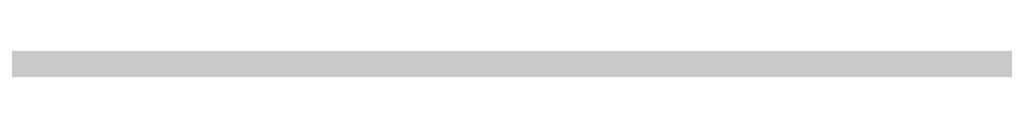
# Model space of a CAD drawing. Units: millimetres. Extents: x 0 to 2267, y 0 to 1823.
# Tile 73 of 256: x 1596.855 to 1600.369, y 1227.284 to 1227.321. Entities that reach past the tile are written whole.
import ezdxf

# ---------------------------------------------------------------- set-up
doc = ezdxf.new("R2010")
doc.units = ezdxf.units.MM
doc.header["$MEASUREMENT"] = 0
doc.layers.add('M-DIMS', color=2, linetype='Continuous', lineweight=25)
doc.layers.add('M-HATC', color=252, linetype='Continuous', lineweight=18)
doc.styles.get("Standard").update_dxf_attribs({"font": 'arial.ttf'})
doc.dimstyles.get("Standard").update_dxf_attribs({"dimtxt": 7, "dimasz": 4, "dimexe": 0.18, "dimexo": 0.0625, "dimgap": 0.09, "dimtad": 0, "dimdec": 0, "dimzin": 0, "dimdsep": 46, "dimtxsty": 'Standard', "dimcen": 0.09, "dimadec": 0, "dimazin": 0, "dimtfac": 1, "dimtdec": 0, "dimtofl": 0, "dimtmove": 0, "dimatfit": 3, "dimfxl": 1, "dimtolj": 1, "dimtzin": 0, "dimarcsym": 0})

# ---------------------------------------------------------------- blocks, each defined once
blk = doc.blocks.new('*D19')
at = {"layer": 'Defpoints', "color": 0, "transparency": 16777216}
for p in [(1605.3399, 1483.3044), (1445.5291, 1333.8851)]:
    blk.add_point(p, dxfattribs=at)
at = {"layer": 'M-DIMS', "color": 0, "lineweight": -2, "transparency": 16777216}
for p, q in [((1605.3399, 1483.2144), (1605.3399, 1483.3944)), ((1605.2499, 1483.3044), (1605.4299, 1483.3044)), ((1366.3244, 1259.8306), (1442.6072, 1331.1532))]:
    blk.add_line(p, q, dxfattribs=at)
at = {"layer": 'M-DIMS', "color": 0, "transparency": 16777216}
blk.add_solid([(1442.1519, 1331.6402), (1443.0625, 1330.6663), (1445.5291, 1333.8851)], dxfattribs=at)
at = {"layer": 'M-DIMS', "color": 0, "transparency": 16777216, "insert": (1349.6425, 1244.2335), "char_height": 7, "attachment_point": 5, "rotation": 43.0753}
blk.add_mtext('\\A1;2X R218.8', dxfattribs=at)

msp = doc.modelspace()

# ---------------------------------------------------------------- hatches: boundary and pattern name
at = {"layer": 'M-HATC'}
h = msp.add_hatch(color=256, dxfattribs=at)
h.dxf.hatch_style = 1
h.paths.add_polyline_path([(2055.771, 1603.062), (1381.0868, 1603.062), (1381.0868, 1598.062), (2055.771, 1598.062)])
h.paths.add_polyline_path([(2055.771, 1598.062), (1381.0868, 1598.062), (1381.0868, 1593.062), (2055.771, 1593.062)])
h.paths.add_polyline_path([(2051.3074, 1536.7609), (1385.5504, 1536.7609), (1385.5504, 1526.7609), (1387.5504, 1526.7609), (1388.5366, 1525.0528), (1385.3319, 1521.2335), (1385.3319, 1521.2226), (2050.2542, 1522.7491), (2048.3212, 1525.0528), (2049.3074, 1526.7609), (2051.3074, 1526.7609)])
edge = h.paths.add_edge_path()
edge.add_arc((1847.5345, 1379.1492), 135, 222.603061, 222.890851, ccw=False)
edge.add_line((1748.1663, 1287.7656), (1683.0921, 1287.7656))
edge.add_arc((1583.7239, 1379.1492), 135, 317.109149, 317.396939, ccw=False)
edge.add_arc((1678.9686, 1290.6707), 5, 222.8909, 317.1091, ccw=False)
edge.add_arc((1774.2133, 1379.1492), 135, 222.603061, 222.890851, ccw=False)
edge.add_line((1674.8451, 1287.7656), (1609.7709, 1287.7656))
edge.add_arc((1510.4027, 1379.1492), 135, 317.109149, 317.396939, ccw=False)
edge.add_arc((1605.6474, 1290.6707), 5, 222.8909, 317.1091, ccw=False)
edge.add_arc((1700.8921, 1379.1492), 135, 222.603061, 222.890851, ccw=False)
edge.add_line((1601.5239, 1287.7656), (1536.4497, 1287.7656))
edge.add_arc((1437.0815, 1379.1492), 135, 317.109149, 317.396939, ccw=False)
edge.add_arc((1532.3262, 1290.6707), 5, 222.8909, 317.1091, ccw=False)
edge.add_arc((1627.5709, 1379.1492), 135, 222.603061, 222.890851, ccw=False)
edge.add_line((1528.2027, 1287.7656), (1505.9289, 1287.7656))
edge.add_spline(control_points=[(1505.9289, 1287.7656), (1504.2622, 1287.7656), (1504.2622, 1282.7656), (1505.9289, 1282.7656)], knot_values=[0, 0, 0, 0, 5, 5, 5, 5], degree=3, periodic=0)
edge.add_line((1505.9289, 1282.7656), (1930.9289, 1282.7656))
edge.add_spline(control_points=[(1930.9289, 1282.7656), (1932.5956, 1282.7656), (1932.5956, 1287.7656), (1930.9289, 1287.7656)], knot_values=[0, 0, 0, 0, 5, 5, 5, 5], degree=3, periodic=0)
edge.add_line((1930.9289, 1287.7656), (1903.0557, 1287.7656))
edge.add_arc((1803.6875, 1379.1492), 135, 317.109149, 317.396939, ccw=False)
edge.add_arc((1898.9322, 1290.6707), 5, 222.8909, 317.1091, ccw=False)
edge.add_arc((1994.1769, 1379.1492), 135, 222.603061, 222.890851, ccw=False)
edge.add_line((1894.8087, 1287.7656), (1829.7345, 1287.7656))
edge.add_arc((1730.3663, 1379.1492), 135, 317.109149, 317.396939, ccw=False)
edge.add_arc((1825.611, 1290.6707), 5, 222.8909, 317.1091, ccw=False)
edge.add_arc((1920.8557, 1379.1492), 135, 222.603061, 222.890851, ccw=False)
edge.add_line((1821.4875, 1287.7656), (1756.4133, 1287.7656))
edge.add_arc((1657.0451, 1379.1492), 135, 317.109149, 317.396939, ccw=False)
edge.add_arc((1752.2898, 1290.6707), 5, 222.8909, 317.1091, ccw=False)
edge = h.paths.add_edge_path()
edge.add_spline(control_points=[(1843.4289, 1227.2475), (1845.0956, 1227.2475), (1845.0956, 1232.2475), (1843.4289, 1232.2475)], knot_values=[0, 0, 0, 0, 5, 5, 5, 5], degree=3, periodic=0)
edge.add_line((1843.4289, 1232.2475), (1593.4289, 1232.2475))
edge.add_spline(control_points=[(1593.4289, 1232.2475), (1591.7622, 1232.2475), (1591.7622, 1227.2475), (1593.4289, 1227.2475)], knot_values=[0, 0, 0, 0, 5, 5, 5, 5], degree=3, periodic=0)
edge.add_line((1593.4289, 1227.2475), (1843.4289, 1227.2475))
h.paths.add_polyline_path([(1905.9289, 1127.4171), (1530.9289, 1127.4171, 0.414214), (1520.9289, 1117.4171), (1530.9289, 1117.4171), (1915.9289, 1117.4171, 0.414214)])
edge = h.paths.add_edge_path()
edge.add_arc((1397.0858, 1498.4078), 12.7299, 90.78215, 190.87871, ccw=False)
edge.add_line((1396.912, 1511.1365), (1428.0097, 1511.3488))
edge.add_line((1428.0097, 1511.3488), (1433.0097, 1511.3488))
edge.add_line((1433.0097, 1511.3488), (1434.439, 1511.3488))
edge.add_arc((1419.474, 1498.0804), 20, 41.561, 74.08211)
edge.add_line((1424.9592, 1517.3135), (1399.9351, 1517.2561))
edge.add_spline(control_points=[(1399.9307, 1517.2561), (1399.884, 1517.2131), (1399.8328, 1517.1689), (1399.7774, 1517.1236)], knot_values=[11.567499, 11.567499, 11.567499, 11.567499, 11.814249, 11.814249, 11.814249, 11.814249], degree=3, periodic=0)
edge.add_spline(control_points=[(1399.6328, 1517.0099), (1399.5831, 1516.9721), (1399.5307, 1516.9338), (1399.4759, 1516.8947)], knot_values=[11.167718, 11.167718, 11.167718, 11.167718, 11.365188, 11.365188, 11.365188, 11.365188], degree=3, periodic=0)
edge.add_spline(control_points=[(1399.3398, 1516.8001), (1399.1514, 1516.6719), (1398.9384, 1516.5377), (1398.704, 1516.3994)], knot_values=[10.376405, 10.376405, 10.376405, 10.376405, 11.00994, 11.00994, 11.00994, 11.00994], degree=3, periodic=0)
edge.add_spline(control_points=[(1398.6572, 1516.3719), (1398.5789, 1516.326), (1398.4983, 1516.2797), (1398.4155, 1516.2331)], knot_values=[10.125175, 10.125175, 10.125175, 10.125175, 10.334406, 10.334406, 10.334406, 10.334406], degree=3, periodic=0)
edge.add_spline(control_points=[(1398.2642, 1516.1487), (1398.196, 1516.1111), (1398.1263, 1516.0732), (1398.0555, 1516.0351)], knot_values=[9.832246, 9.832246, 9.832246, 9.832246, 9.999658, 9.999658, 9.999658, 9.999658], degree=3, periodic=0)
edge.add_spline(control_points=[(1397.9987, 1516.0048), (1397.7312, 1515.8621), (1397.446, 1515.7171), (1397.1466, 1515.5714)], knot_values=[9.161808, 9.161808, 9.161808, 9.161808, 9.787769, 9.787769, 9.787769, 9.787769], degree=3, periodic=0)
edge.add_spline(control_points=[(1397.1466, 1515.5714), (1396.8418, 1515.423), (1396.5222, 1515.274), (1396.1914, 1515.1262)], knot_values=[8.524455, 8.524455, 8.524455, 8.524455, 9.161808, 9.161808, 9.161808, 9.161808], degree=3, periodic=0)
edge.add_spline(control_points=[(1396.0777, 1515.0756), (1395.9854, 1515.0348), (1395.8922, 1514.994), (1395.7983, 1514.9534)], knot_values=[8.275193, 8.275193, 8.275193, 8.275193, 8.451726, 8.451726, 8.451726, 8.451726], degree=3, periodic=0)
edge.add_spline(control_points=[(1395.6018, 1514.8691), (1395.4997, 1514.8257), (1395.3968, 1514.7824), (1395.2932, 1514.7394)], knot_values=[7.962917, 7.962917, 7.962917, 7.962917, 8.152764, 8.152764, 8.152764, 8.152764], degree=3, periodic=0)
edge.add_spline(control_points=[(1395.2116, 1514.7057), (1394.8278, 1514.5475), (1394.4345, 1514.3929), (1394.0364, 1514.2442)], knot_values=[7.21254, 7.21254, 7.21254, 7.21254, 7.913148, 7.913148, 7.913148, 7.913148], degree=3, periodic=0)
edge.add_spline(control_points=[(1394.0364, 1514.2442), (1393.7076, 1514.1214), (1393.3754, 1514.0027), (1393.0427, 1513.8895)], knot_values=[6.633733, 6.633733, 6.633733, 6.633733, 7.21254, 7.21254, 7.21254, 7.21254], degree=3, periodic=0)
edge.add_spline(control_points=[(1392.8214, 1513.815), (1392.7198, 1513.7812), (1392.6181, 1513.7479), (1392.5166, 1513.7152)], knot_values=[6.328796, 6.328796, 6.328796, 6.328796, 6.505493, 6.505493, 6.505493, 6.505493], degree=3, periodic=0)
edge.add_spline(control_points=[(1392.5166, 1513.7152), (1392.3187, 1513.6515), (1392.1212, 1513.59), (1391.9244, 1513.531)], knot_values=[5.984605, 5.984605, 5.984605, 5.984605, 6.328796, 6.328796, 6.328796, 6.328796], degree=3, periodic=0)
edge.add_spline(control_points=[(1391.7915, 1513.4915), (1391.3122, 1513.3501), (1390.8384, 1513.2239), (1390.3784, 1513.1171)], knot_values=[5.066697, 5.066697, 5.066697, 5.066697, 5.907055, 5.907055, 5.907055, 5.907055], degree=3, periodic=0)
edge.add_spline(control_points=[(1390.3784, 1513.1171), (1390.1797, 1513.071), (1389.9836, 1513.0284), (1389.7907, 1512.9899)], knot_values=[4.70367, 4.70367, 4.70367, 4.70367, 5.066695, 5.066695, 5.066695, 5.066695], degree=3, periodic=0)
edge.add_spline(control_points=[(1389.422, 1512.9204), (1389.2459, 1512.8892), (1389.0729, 1512.8617), (1388.9036, 1512.8381)], knot_values=[4.130571, 4.130571, 4.130571, 4.130571, 4.469816, 4.469816, 4.469816, 4.469816], degree=3, periodic=0)
edge.add_spline(control_points=[(1388.9036, 1512.8381), (1388.591, 1512.7946), (1388.2911, 1512.7644), (1388.0071, 1512.7494)], knot_values=[3.504031, 3.504031, 3.504031, 3.504031, 4.130571, 4.130571, 4.130571, 4.130571], degree=3, periodic=0)
edge.add_spline(control_points=[(1387.9356, 1512.7459), (1387.8538, 1512.7423), (1387.7733, 1512.74), (1387.6944, 1512.739)], knot_values=[3.268866, 3.268866, 3.268866, 3.268866, 3.451164, 3.451164, 3.451164, 3.451164], degree=3, periodic=0)
edge.add_spline(control_points=[(1387.3351, 1512.7443), (1387.2076, 1512.7499), (1387.0847, 1512.7597), (1386.967, 1512.7739)], knot_values=[2.670686, 2.670686, 2.670686, 2.670686, 2.984, 2.984, 2.984, 2.984], degree=3, periodic=0)
edge.add_spline(control_points=[(1386.8327, 1512.7922), (1386.8209, 1512.7941), (1386.8092, 1512.7959), (1386.7975, 1512.7979)], knot_values=[2.516981, 2.516981, 2.516981, 2.516981, 2.549528, 2.549528, 2.549528, 2.549528], degree=3, periodic=0)
edge.add_spline(control_points=[(1386.4526, 1512.8735), (1386.4257, 1512.881), (1386.3993, 1512.889), (1386.3733, 1512.8972)], knot_values=[2.095869, 2.095869, 2.095869, 2.095869, 2.17941, 2.17941, 2.17941, 2.17941], degree=3, periodic=0)
edge.add_spline(control_points=[(1386.0691, 1513.0189), (1386.0634, 1513.0217), (1386.0577, 1513.0246), (1386.052, 1513.0275)], knot_values=[1.72453, 1.72453, 1.72453, 1.72453, 1.745933, 1.745933, 1.745933, 1.745933], degree=3, periodic=0)
edge.add_arc((1399.474, 1498.0804), 20, 131.82432, 180)
edge.add_arc((1630.3336, 1505.5484), 250.9708, 181.705176, 236.427975)
edge.add_arc((1605.3399, 1483.3044), 218.7822, 238.660829, 243.34961)
edge.add_arc((1647.0911, 1510.3592), 262.8986, 183.129836, 237.853442, ccw=False)
h.paths.add_polyline_path([(1406.5369, 1391.9644, 0.149382), (1491.5506, 1296.4418, -0.129517)], flags=17)
edge = h.paths.add_edge_path()
edge.add_arc((2037.3838, 1498.0804), 20, 0, 48.26587)
edge.add_spline(control_points=[(2050.6973, 1513.0052), (2050.6512, 1512.9847), (2050.6034, 1512.9655), (2050.5539, 1512.9477)], knot_values=[1.835652, 1.835652, 1.835652, 1.835652, 2.000781, 2.000781, 2.000781, 2.000781], degree=3, periodic=0)
edge.add_spline(control_points=[(2050.4616, 1512.9166), (2050.479, 1512.9221), (2050.4963, 1512.9277), (2050.5133, 1512.9335)], knot_values=[2.045477, 2.045477, 2.045477, 2.045477, 2.101389, 2.101389, 2.101389, 2.101389], degree=3, periodic=0)
edge.add_spline(control_points=[(2050.129, 1512.8342), (2050.1984, 1512.8473), (2050.2657, 1512.8623), (2050.3308, 1512.8792)], knot_values=[2.237629, 2.237629, 2.237629, 2.237629, 2.435841, 2.435841, 2.435841, 2.435841], degree=3, periodic=0)
edge.add_spline(control_points=[(2050.0946, 1512.8278), (2050.1061, 1512.8299), (2050.1176, 1512.832), (2050.129, 1512.8342)], knot_values=[2.435841, 2.435841, 2.435841, 2.435841, 2.468321, 2.468321, 2.468321, 2.468321], degree=3, periodic=0)
edge.add_spline(control_points=[(2049.7843, 1512.7851), (2049.8552, 1512.7922), (2049.9243, 1512.8008), (2049.9917, 1512.8109)], knot_values=[2.563852, 2.563852, 2.563852, 2.563852, 2.748541, 2.748541, 2.748541, 2.748541], degree=3, periodic=0)
edge.add_spline(control_points=[(2049.4052, 1512.7617), (2049.5364, 1512.7653), (2049.6629, 1512.773), (2049.7843, 1512.7851)], knot_values=[2.748541, 2.748541, 2.748541, 2.748541, 3.064882, 3.064882, 3.064882, 3.064882], degree=3, periodic=0)
edge.add_spline(control_points=[(2049.1698, 1512.7597), (2049.2336, 1512.7591), (2049.2965, 1512.7594), (2049.3584, 1512.7606)], knot_values=[3.102309, 3.102309, 3.102309, 3.102309, 3.2503, 3.2503, 3.2503, 3.2503], degree=3, periodic=0)
edge.add_spline(control_points=[(2048.8573, 1512.7691), (2048.9638, 1512.7638), (2049.068, 1512.7606), (2049.1698, 1512.7597)], knot_values=[3.2503, 3.2503, 3.2503, 3.2503, 3.486069, 3.486069, 3.486069, 3.486069], degree=3, periodic=0)
edge.add_spline(control_points=[(2048.6924, 1512.7789), (2048.3729, 1512.8009), (2048.0345, 1512.8411), (2047.6817, 1512.897)], knot_values=[3.606429, 3.606429, 3.606429, 3.606429, 4.2989, 4.2989, 4.2989, 4.2989], degree=3, periodic=0)
edge.add_spline(control_points=[(2047.6817, 1512.897), (2047.5458, 1512.9185), (2047.4077, 1512.9424), (2047.2678, 1512.9685)], knot_values=[4.2989, 4.2989, 4.2989, 4.2989, 4.565769, 4.565769, 4.565769, 4.565769], degree=3, periodic=0)
edge.add_spline(control_points=[(2047.2678, 1512.9685), (2047.1449, 1512.9914), (2047.0207, 1513.016), (2046.8951, 1513.0422)], knot_values=[4.565769, 4.565769, 4.565769, 4.565769, 4.799971, 4.799971, 4.799971, 4.799971], degree=3, periodic=0)
edge.add_spline(control_points=[(2046.8951, 1513.0422), (2046.5286, 1513.1188), (2046.1513, 1513.209), (2045.7676, 1513.3107)], knot_values=[4.799971, 4.799971, 4.799971, 4.799971, 5.483718, 5.483718, 5.483718, 5.483718], degree=3, periodic=0)
edge.add_spline(control_points=[(2045.7676, 1513.3107), (2045.3724, 1513.4154), (2044.9704, 1513.5322), (2044.5662, 1513.6588)], knot_values=[5.483718, 5.483718, 5.483718, 5.483718, 6.187866, 6.187866, 6.187866, 6.187866], degree=3, periodic=0)
edge.add_spline(control_points=[(2044.5662, 1513.6588), (2044.4149, 1513.7061), (2044.2633, 1513.7549), (2044.1116, 1513.8048)], knot_values=[6.187866, 6.187866, 6.187866, 6.187866, 6.451551, 6.451551, 6.451551, 6.451551], degree=3, periodic=0)
edge.add_spline(control_points=[(2044.1116, 1513.8048), (2043.9967, 1513.8427), (2043.8817, 1513.8813), (2043.7668, 1513.9205)], knot_values=[6.451551, 6.451551, 6.451551, 6.451551, 6.651434, 6.651434, 6.651434, 6.651434], degree=3, periodic=0)
edge.add_spline(control_points=[(2043.7668, 1513.9205), (2043.3716, 1514.0554), (2042.9774, 1514.1979), (2042.5886, 1514.3458)], knot_values=[6.651434, 6.651434, 6.651434, 6.651434, 7.338879, 7.338879, 7.338879, 7.338879], degree=3, periodic=0)
edge.add_spline(control_points=[(2042.5886, 1514.3458), (2042.1643, 1514.5071), (2041.7465, 1514.6749), (2041.3409, 1514.846)], knot_values=[7.338879, 7.338879, 7.338879, 7.338879, 8.089209, 8.089209, 8.089209, 8.089209], degree=3, periodic=0)
edge.add_spline(control_points=[(2041.3409, 1514.846), (2041.1028, 1514.9465), (2040.869, 1515.0481), (2040.6405, 1515.1502)], knot_values=[8.089209, 8.089209, 8.089209, 8.089209, 8.529587, 8.529587, 8.529587, 8.529587], degree=3, periodic=0)
edge.add_spline(control_points=[(2040.51, 1515.2089), (2040.0824, 1515.4022), (2039.6747, 1515.5971), (2039.295, 1515.7894)], knot_values=[8.613818, 8.613818, 8.613818, 8.613818, 9.44571, 9.44571, 9.44571, 9.44571], degree=3, periodic=0)
edge.add_spline(control_points=[(2039.295, 1515.7894), (2039.0618, 1515.9075), (2038.8391, 1516.0246), (2038.6288, 1516.1398)], knot_values=[9.44571, 9.44571, 9.44571, 9.44571, 9.956404, 9.956404, 9.956404, 9.956404], degree=3, periodic=0)
edge.add_spline(control_points=[(2038.6288, 1516.1398), (2038.5187, 1516.2001), (2038.4121, 1516.2598), (2038.309, 1516.3189)], knot_values=[9.956404, 9.956404, 9.956404, 9.956404, 10.223542, 10.223542, 10.223542, 10.223542], degree=3, periodic=0)
edge.add_spline(control_points=[(2038.309, 1516.3189), (2038.2138, 1516.3735), (2038.1216, 1516.4276), (2038.0328, 1516.481)], knot_values=[10.223542, 10.223542, 10.223542, 10.223542, 10.47051, 10.47051, 10.47051, 10.47051], degree=3, periodic=0)
edge.add_spline(control_points=[(2038.0328, 1516.481), (2037.7855, 1516.6296), (2037.5639, 1516.773), (2037.3722, 1516.909)], knot_values=[10.47051, 10.47051, 10.47051, 10.47051, 11.15767, 11.15767, 11.15767, 11.15767], degree=3, periodic=0)
edge.add_spline(control_points=[(2037.3722, 1516.909), (2037.2789, 1516.9752), (2037.1927, 1517.0396), (2037.1142, 1517.102)], knot_values=[11.15767, 11.15767, 11.15767, 11.15767, 11.49227, 11.49227, 11.49227, 11.49227], degree=3, periodic=0)
edge.add_spline(control_points=[(2036.8564, 1517.3259), (2036.9148, 1517.2692), (2036.9814, 1517.2103), (2037.0557, 1517.1492)], knot_values=[11.577341, 11.577341, 11.577341, 11.577341, 11.91035, 11.91035, 11.91035, 11.91035], degree=3, periodic=0)
edge.add_spline(control_points=[(2036.8074, 1517.3748), (2036.823, 1517.3587), (2036.8393, 1517.3424), (2036.8564, 1517.3259)], knot_values=[11.91035, 11.91035, 11.91035, 11.91035, 12.007402, 12.007402, 12.007402, 12.007402], degree=3, periodic=0)
edge.add_spline(control_points=[(2036.7017, 1517.494), (2036.7104, 1517.483), (2036.7196, 1517.4719), (2036.7291, 1517.4606)], knot_values=[12.184155, 12.184155, 12.184155, 12.184155, 12.255409, 12.255409, 12.255409, 12.255409], degree=3, periodic=0)
edge.add_spline(control_points=[(2036.6159, 1517.6205), (2036.62, 1517.613), (2036.6243, 1517.6055), (2036.6289, 1517.5979)], knot_values=[12.487913, 12.487913, 12.487913, 12.487913, 12.541035, 12.541035, 12.541035, 12.541035], degree=3, periodic=0)
edge.add_spline(control_points=[(2036.5635, 1517.786), (2036.5637, 1517.7794), (2036.5642, 1517.7726), (2036.565, 1517.7658)], knot_values=[12.911761, 12.911761, 12.911761, 12.911761, 12.968286, 12.968286, 12.968286, 12.968286], degree=3, periodic=0)
edge.add_spline(control_points=[(2036.6166, 1517.9304), (2036.6125, 1517.9259), (2036.6086, 1517.9212), (2036.6049, 1517.9165)], knot_values=[13.382527, 13.382527, 13.382527, 13.382527, 13.433791, 13.433791, 13.433791, 13.433791], degree=3, periodic=0)
edge.add_spline(control_points=[(2036.749, 1518.017), (2036.7361, 1518.0116), (2036.7239, 1518.006), (2036.7124, 1518.0002)], knot_values=[13.726299, 13.726299, 13.726299, 13.726299, 13.809928, 13.809928, 13.809928, 13.809928], degree=3, periodic=0)
edge.add_spline(control_points=[(2036.8604, 1518.0528), (2036.8386, 1518.0474), (2036.8181, 1518.0416), (2036.7988, 1518.0353)], knot_values=[13.910887, 13.910887, 13.910887, 13.910887, 14.02153, 14.02153, 14.02153, 14.02153], degree=3, periodic=0)
edge.add_line((2036.9639, 1518.0804), (2032.3838, 1518.0804))
edge.add_line((2032.3838, 1518.0804), (2027.3838, 1518.0804))
edge.add_line((2027.3838, 1518.0804), (2022.3838, 1518.0804))
edge.add_line((2022.3838, 1518.0804), (2017.3838, 1518.0804))
edge.add_arc((2017.3838, 1498.0804), 20, 90, 138.439)
edge.add_line((2002.4188, 1511.3488), (2003.8481, 1511.3488))
edge.add_line((2003.8481, 1511.3488), (2008.8481, 1511.3488))
edge.add_line((2008.8481, 1511.3488), (2039.772, 1511.1377))
edge.add_arc((2039.772, 1498.4078), 12.7299, -10.87871, 90, ccw=False)
edge.add_arc((1789.7668, 1510.3592), 262.8986, 302.146558, 356.870164, ccw=False)
edge.add_arc((1831.5179, 1483.3044), 218.7822, 296.65039, 301.339171)
edge.add_arc((1806.5242, 1505.5484), 250.9708, 303.572025, 358.294824)
h.paths.add_polyline_path([(2030.321, 1391.9644, -0.129517), (1945.3072, 1296.4418, 0.149382)], flags=17)
edge = h.paths.add_edge_path()
edge.add_spline(control_points=[(2037.2464, 1518.0821), (2037.2898, 1518.081), (2037.3355, 1518.0804), (2037.3838, 1518.0804)], knot_values=[0.000012, 0.000012, 0.000012, 0.000012, 0.144754, 0.144754, 0.144754, 0.144754], degree=3, periodic=0)
edge.add_line((2037.3357, 1518.0804), (2037.0096, 1518.0804))
edge.add_spline(control_points=[(2037.0096, 1518.0804), (2036.9822, 1518.0768), (2036.956, 1518.0727), (2036.9312, 1518.0681)], knot_values=[14.13465, 14.13465, 14.13465, 14.13465, 14.247197, 14.247197, 14.247197, 14.247197], degree=3, periodic=0)
edge.add_spline(control_points=[(2036.9312, 1518.0681), (2036.9276, 1518.0674), (2036.9241, 1518.0667), (2036.9205, 1518.0661)], knot_values=[14.118315, 14.118315, 14.118315, 14.118315, 14.13465, 14.13465, 14.13465, 14.13465], degree=3, periodic=0)
edge.add_spline(control_points=[(2036.9205, 1518.0661), (2036.9118, 1518.0644), (2036.9032, 1518.0626), (2036.8948, 1518.0608)], knot_values=[14.078086, 14.078086, 14.078086, 14.078086, 14.118315, 14.118315, 14.118315, 14.118315], degree=3, periodic=0)
edge.add_spline(control_points=[(2036.8948, 1518.0608), (2036.883, 1518.0583), (2036.8716, 1518.0556), (2036.8604, 1518.0528)], knot_values=[14.02153, 14.02153, 14.02153, 14.02153, 14.078086, 14.078086, 14.078086, 14.078086], degree=3, periodic=0)
edge.add_spline(control_points=[(2036.8604, 1518.0528), (2036.8386, 1518.0474), (2036.8181, 1518.0416), (2036.7988, 1518.0353)], knot_values=[13.910887, 13.910887, 13.910887, 13.910887, 14.02153, 14.02153, 14.02153, 14.02153], degree=3, periodic=0)
edge.add_spline(control_points=[(2036.7988, 1518.0353), (2036.7981, 1518.035), (2036.7974, 1518.0348), (2036.7967, 1518.0346)], knot_values=[13.906906, 13.906906, 13.906906, 13.906906, 13.910887, 13.910887, 13.910887, 13.910887], degree=3, periodic=0)
edge.add_spline(control_points=[(2036.7967, 1518.0346), (2036.7882, 1518.0318), (2036.7799, 1518.0289), (2036.7719, 1518.0259)], knot_values=[13.857826, 13.857826, 13.857826, 13.857826, 13.906906, 13.906906, 13.906906, 13.906906], degree=3, periodic=0)
edge.add_spline(control_points=[(2036.7719, 1518.0259), (2036.764, 1518.023), (2036.7564, 1518.02), (2036.749, 1518.017)], knot_values=[13.809928, 13.809928, 13.809928, 13.809928, 13.857826, 13.857826, 13.857826, 13.857826], degree=3, periodic=0)
edge.add_spline(control_points=[(2036.749, 1518.017), (2036.7361, 1518.0116), (2036.7239, 1518.006), (2036.7124, 1518.0002)], knot_values=[13.726299, 13.726299, 13.726299, 13.726299, 13.809928, 13.809928, 13.809928, 13.809928], degree=3, periodic=0)
edge.add_spline(control_points=[(2036.7124, 1518.0002), (2036.7121, 1518), (2036.7118, 1517.9999), (2036.7115, 1517.9997)], knot_values=[13.723993, 13.723993, 13.723993, 13.723993, 13.726299, 13.726299, 13.726299, 13.726299], degree=3, periodic=0)
edge.add_spline(control_points=[(2036.7115, 1517.9997), (2036.7063, 1517.9971), (2036.7013, 1517.9944), (2036.6965, 1517.9917)], knot_values=[13.686536, 13.686536, 13.686536, 13.686536, 13.723993, 13.723993, 13.723993, 13.723993], degree=3, periodic=0)
edge.add_spline(control_points=[(2036.6965, 1517.9917), (2036.6919, 1517.9891), (2036.6874, 1517.9865), (2036.6831, 1517.9839)], knot_values=[13.651251, 13.651251, 13.651251, 13.651251, 13.686536, 13.686536, 13.686536, 13.686536], degree=3, periodic=0)
edge.add_spline(control_points=[(2036.6831, 1517.9839), (2036.6764, 1517.9798), (2036.67, 1517.9757), (2036.6639, 1517.9714)], knot_values=[13.596804, 13.596804, 13.596804, 13.596804, 13.651251, 13.651251, 13.651251, 13.651251], degree=3, periodic=0)
edge.add_spline(control_points=[(2036.6639, 1517.9714), (2036.6636, 1517.9712), (2036.6633, 1517.9709), (2036.6629, 1517.9707)], knot_values=[13.593956, 13.593956, 13.593956, 13.593956, 13.596804, 13.596804, 13.596804, 13.596804], degree=3, periodic=0)
edge.add_spline(control_points=[(2036.6629, 1517.9707), (2036.6603, 1517.9689), (2036.6577, 1517.967), (2036.6552, 1517.9651)], knot_values=[13.570322, 13.570322, 13.570322, 13.570322, 13.593956, 13.593956, 13.593956, 13.593956], degree=3, periodic=0)
edge.add_spline(control_points=[(2036.6552, 1517.9651), (2036.6525, 1517.9631), (2036.6499, 1517.9611), (2036.6474, 1517.9591)], knot_values=[13.545477, 13.545477, 13.545477, 13.545477, 13.570322, 13.570322, 13.570322, 13.570322], degree=3, periodic=0)
edge.add_spline(control_points=[(2036.6474, 1517.9591), (2036.6472, 1517.9589), (2036.6471, 1517.9588), (2036.6469, 1517.9587)], knot_values=[13.543931, 13.543931, 13.543931, 13.543931, 13.545477, 13.545477, 13.545477, 13.545477], degree=3, periodic=0)
edge.add_spline(control_points=[(2036.6469, 1517.9587), (2036.6412, 1517.9541), (2036.6358, 1517.9494), (2036.6307, 1517.9447)], knot_values=[13.488237, 13.488237, 13.488237, 13.488237, 13.543931, 13.543931, 13.543931, 13.543931], degree=3, periodic=0)
edge.add_spline(control_points=[(2036.6307, 1517.9447), (2036.6282, 1517.9423), (2036.6257, 1517.9399), (2036.6233, 1517.9374)], knot_values=[13.460307, 13.460307, 13.460307, 13.460307, 13.488237, 13.488237, 13.488237, 13.488237], degree=3, periodic=0)
edge.add_spline(control_points=[(2036.6233, 1517.9374), (2036.6215, 1517.9356), (2036.6198, 1517.9338), (2036.6181, 1517.932)], knot_values=[13.439712, 13.439712, 13.439712, 13.439712, 13.460307, 13.460307, 13.460307, 13.460307], degree=3, periodic=0)
edge.add_spline(control_points=[(2036.6181, 1517.932), (2036.6176, 1517.9315), (2036.6171, 1517.9309), (2036.6166, 1517.9304)], knot_values=[13.433791, 13.433791, 13.433791, 13.433791, 13.439712, 13.439712, 13.439712, 13.439712], degree=3, periodic=0)
edge.add_spline(control_points=[(2036.6166, 1517.9304), (2036.6125, 1517.9259), (2036.6086, 1517.9212), (2036.6049, 1517.9165)], knot_values=[13.382527, 13.382527, 13.382527, 13.382527, 13.433791, 13.433791, 13.433791, 13.433791], degree=3, periodic=0)
edge.add_spline(control_points=[(2036.6049, 1517.9165), (2036.6026, 1517.9135), (2036.6004, 1517.9104), (2036.5982, 1517.9074)], knot_values=[13.350017, 13.350017, 13.350017, 13.350017, 13.382527, 13.382527, 13.382527, 13.382527], degree=3, periodic=0)
edge.add_spline(control_points=[(2036.5982, 1517.9074), (2036.5972, 1517.9059), (2036.5962, 1517.9043), (2036.5952, 1517.9028)], knot_values=[13.333922, 13.333922, 13.333922, 13.333922, 13.350017, 13.350017, 13.350017, 13.350017], degree=3, periodic=0)
edge.add_spline(control_points=[(2036.5952, 1517.9028), (2036.5945, 1517.9018), (2036.5939, 1517.9009), (2036.5933, 1517.8999)], knot_values=[13.323828, 13.323828, 13.323828, 13.323828, 13.333922, 13.333922, 13.333922, 13.333922], degree=3, periodic=0)
edge.add_spline(control_points=[(2036.5933, 1517.8999), (2036.5905, 1517.8955), (2036.5879, 1517.8909), (2036.5855, 1517.8864)], knot_values=[13.277545, 13.277545, 13.277545, 13.277545, 13.323828, 13.323828, 13.323828, 13.323828], degree=3, periodic=0)
edge.add_spline(control_points=[(2036.5855, 1517.8864), (2036.5836, 1517.8827), (2036.5817, 1517.8789), (2036.5801, 1517.8751)], knot_values=[13.240119, 13.240119, 13.240119, 13.240119, 13.277545, 13.277545, 13.277545, 13.277545], degree=3, periodic=0)
edge.add_spline(control_points=[(2036.5801, 1517.8751), (2036.5795, 1517.8739), (2036.579, 1517.8727), (2036.5785, 1517.8715)], knot_values=[13.228211, 13.228211, 13.228211, 13.228211, 13.240119, 13.240119, 13.240119, 13.240119], degree=3, periodic=0)
edge.add_spline(control_points=[(2036.5785, 1517.8715), (2036.578, 1517.8702), (2036.5774, 1517.869), (2036.5769, 1517.8677)], knot_values=[13.215717, 13.215717, 13.215717, 13.215717, 13.228211, 13.228211, 13.228211, 13.228211], degree=3, periodic=0)
edge.add_spline(control_points=[(2036.5769, 1517.8677), (2036.5755, 1517.864), (2036.5741, 1517.8603), (2036.5729, 1517.8565)], knot_values=[13.179847, 13.179847, 13.179847, 13.179847, 13.215717, 13.215717, 13.215717, 13.215717], degree=3, periodic=0)
edge.add_spline(control_points=[(2036.5729, 1517.8565), (2036.5713, 1517.8515), (2036.5699, 1517.8464), (2036.5687, 1517.8413)], knot_values=[13.132017, 13.132017, 13.132017, 13.132017, 13.179847, 13.179847, 13.179847, 13.179847], degree=3, periodic=0)
edge.add_spline(control_points=[(2036.5687, 1517.8413), (2036.5684, 1517.8402), (2036.5682, 1517.8392), (2036.568, 1517.8382)], knot_values=[13.122482, 13.122482, 13.122482, 13.122482, 13.132017, 13.132017, 13.132017, 13.132017], degree=3, periodic=0)
edge.add_spline(control_points=[(2036.568, 1517.8382), (2036.5676, 1517.8363), (2036.5672, 1517.8345), (2036.5669, 1517.8327)], knot_values=[13.105592, 13.105592, 13.105592, 13.105592, 13.122482, 13.122482, 13.122482, 13.122482], degree=3, periodic=0)
edge.add_spline(control_points=[(2036.5669, 1517.8327), (2036.5662, 1517.8292), (2036.5657, 1517.8257), (2036.5652, 1517.8222)], knot_values=[13.074063, 13.074063, 13.074063, 13.074063, 13.105592, 13.105592, 13.105592, 13.105592], degree=3, periodic=0)
edge.add_spline(control_points=[(2036.5652, 1517.8222), (2036.5652, 1517.8222), (2036.5652, 1517.8222), (2036.5652, 1517.8222)], knot_values=[13.074043, 13.074043, 13.074043, 13.074043, 13.074063, 13.074063, 13.074063, 13.074063], degree=3, periodic=0)
edge.add_spline(control_points=[(2036.5652, 1517.8222), (2036.5644, 1517.8164), (2036.5639, 1517.8106), (2036.5636, 1517.8046)], knot_values=[13.021884, 13.021884, 13.021884, 13.021884, 13.074043, 13.074043, 13.074043, 13.074043], degree=3, periodic=0)
edge.add_spline(control_points=[(2036.5636, 1517.8046), (2036.5636, 1517.804), (2036.5636, 1517.8034), (2036.5635, 1517.8028)], knot_values=[13.01674, 13.01674, 13.01674, 13.01674, 13.021884, 13.021884, 13.021884, 13.021884], degree=3, periodic=0)
edge.add_spline(control_points=[(2036.5635, 1517.8028), (2036.5634, 1517.8005), (2036.5634, 1517.7982), (2036.5634, 1517.7958)], knot_values=[12.996438, 12.996438, 12.996438, 12.996438, 13.01674, 13.01674, 13.01674, 13.01674], degree=3, periodic=0)
edge.add_spline(control_points=[(2036.5634, 1517.7958), (2036.5633, 1517.7926), (2036.5634, 1517.7893), (2036.5635, 1517.786)], knot_values=[12.968286, 12.968286, 12.968286, 12.968286, 12.996438, 12.996438, 12.996438, 12.996438], degree=3, periodic=0)
edge.add_spline(control_points=[(2036.5635, 1517.786), (2036.5637, 1517.7794), (2036.5642, 1517.7726), (2036.565, 1517.7658)], knot_values=[12.911761, 12.911761, 12.911761, 12.911761, 12.968286, 12.968286, 12.968286, 12.968286], degree=3, periodic=0)
edge.add_spline(control_points=[(2036.565, 1517.7658), (2036.565, 1517.7657), (2036.565, 1517.7656), (2036.565, 1517.7656)], knot_values=[12.911017, 12.911017, 12.911017, 12.911017, 12.911761, 12.911761, 12.911761, 12.911761], degree=3, periodic=0)
edge.add_spline(control_points=[(2036.565, 1517.7656), (2036.5654, 1517.7625), (2036.5658, 1517.7593), (2036.5663, 1517.7562)], knot_values=[12.88528, 12.88528, 12.88528, 12.88528, 12.911017, 12.911017, 12.911017, 12.911017], degree=3, periodic=0)
edge.add_spline(control_points=[(2036.5663, 1517.7562), (2036.5667, 1517.7534), (2036.5672, 1517.7506), (2036.5677, 1517.7478)], knot_values=[12.862519, 12.862519, 12.862519, 12.862519, 12.88528, 12.88528, 12.88528, 12.88528], degree=3, periodic=0)
edge.add_spline(control_points=[(2036.5677, 1517.7478), (2036.5678, 1517.7474), (2036.5679, 1517.7469), (2036.568, 1517.7465)], knot_values=[12.858885, 12.858885, 12.858885, 12.858885, 12.862519, 12.862519, 12.862519, 12.862519], degree=3, periodic=0)
edge.add_spline(control_points=[(2036.568, 1517.7465), (2036.5692, 1517.7399), (2036.5707, 1517.7332), (2036.5724, 1517.7264)], knot_values=[12.8053, 12.8053, 12.8053, 12.8053, 12.858885, 12.858885, 12.858885, 12.858885], degree=3, periodic=0)
edge.add_spline(control_points=[(2036.5724, 1517.7264), (2036.5734, 1517.7226), (2036.5745, 1517.7187), (2036.5756, 1517.7149)], knot_values=[12.775176, 12.775176, 12.775176, 12.775176, 12.8053, 12.8053, 12.8053, 12.8053], degree=3, periodic=0)
edge.add_spline(control_points=[(2036.5756, 1517.7149), (2036.5763, 1517.7125), (2036.577, 1517.7102), (2036.5778, 1517.7078)], knot_values=[12.756759, 12.756759, 12.756759, 12.756759, 12.775176, 12.775176, 12.775176, 12.775176], degree=3, periodic=0)
edge.add_spline(control_points=[(2036.5778, 1517.7078), (2036.5781, 1517.7067), (2036.5784, 1517.7057), (2036.5787, 1517.7047)], knot_values=[12.748742, 12.748742, 12.748742, 12.748742, 12.756759, 12.756759, 12.756759, 12.756759], degree=3, periodic=0)
edge.add_spline(control_points=[(2036.5787, 1517.7047), (2036.5808, 1517.6983), (2036.5831, 1517.6919), (2036.5856, 1517.6854)], knot_values=[12.69959, 12.69959, 12.69959, 12.69959, 12.748742, 12.748742, 12.748742, 12.748742], degree=3, periodic=0)
edge.add_spline(control_points=[(2036.5856, 1517.6854), (2036.5876, 1517.68), (2036.5898, 1517.6746), (2036.5921, 1517.6692)], knot_values=[12.659038, 12.659038, 12.659038, 12.659038, 12.69959, 12.69959, 12.69959, 12.69959], degree=3, periodic=0)
edge.add_spline(control_points=[(2036.5921, 1517.6692), (2036.594, 1517.6648), (2036.5959, 1517.6605), (2036.5979, 1517.6561)], knot_values=[12.626806, 12.626806, 12.626806, 12.626806, 12.659038, 12.659038, 12.659038, 12.659038], degree=3, periodic=0)
edge.add_spline(control_points=[(2036.5979, 1517.6561), (2036.5984, 1517.6551), (2036.5989, 1517.6541), (2036.5993, 1517.6531)], knot_values=[12.619394, 12.619394, 12.619394, 12.619394, 12.626806, 12.626806, 12.626806, 12.626806], degree=3, periodic=0)
edge.add_spline(control_points=[(2036.5993, 1517.6531), (2036.6043, 1517.6424), (2036.6099, 1517.6315), (2036.6159, 1517.6205)], knot_values=[12.541039, 12.541039, 12.541039, 12.541039, 12.619394, 12.619394, 12.619394, 12.619394], degree=3, periodic=0)
edge.add_spline(control_points=[(2036.6159, 1517.6205), (2036.6159, 1517.6205), (2036.6159, 1517.6205), (2036.6159, 1517.6205)], knot_values=[12.541035, 12.541035, 12.541035, 12.541035, 12.541039, 12.541039, 12.541039, 12.541039], degree=3, periodic=0)
edge.add_spline(control_points=[(2036.6159, 1517.6205), (2036.62, 1517.613), (2036.6243, 1517.6055), (2036.6289, 1517.5979)], knot_values=[12.487913, 12.487913, 12.487913, 12.487913, 12.541035, 12.541035, 12.541035, 12.541035], degree=3, periodic=0)
edge.add_spline(control_points=[(2036.6289, 1517.5979), (2036.6326, 1517.5916), (2036.6365, 1517.5853), (2036.6406, 1517.5789)], knot_values=[12.443982, 12.443982, 12.443982, 12.443982, 12.487913, 12.487913, 12.487913, 12.487913], degree=3, periodic=0)
edge.add_spline(control_points=[(2036.6406, 1517.5789), (2036.6414, 1517.5776), (2036.6423, 1517.5763), (2036.6431, 1517.5749)], knot_values=[12.434996, 12.434996, 12.434996, 12.434996, 12.443982, 12.443982, 12.443982, 12.443982], degree=3, periodic=0)
edge.add_spline(control_points=[(2036.6431, 1517.5749), (2036.6531, 1517.5596), (2036.6639, 1517.5439), (2036.6756, 1517.528)], knot_values=[12.329647, 12.329647, 12.329647, 12.329647, 12.434996, 12.434996, 12.434996, 12.434996], degree=3, periodic=0)
edge.add_spline(control_points=[(2036.6756, 1517.528), (2036.6839, 1517.5168), (2036.6925, 1517.5055), (2036.7017, 1517.494)], knot_values=[12.255409, 12.255409, 12.255409, 12.255409, 12.329647, 12.329647, 12.329647, 12.329647], degree=3, periodic=0)
edge.add_spline(control_points=[(2036.7017, 1517.494), (2036.7104, 1517.483), (2036.7196, 1517.4719), (2036.7291, 1517.4606)], knot_values=[12.184155, 12.184155, 12.184155, 12.184155, 12.255409, 12.255409, 12.255409, 12.255409], degree=3, periodic=0)
edge.add_spline(control_points=[(2036.7291, 1517.4606), (2036.7436, 1517.4435), (2036.759, 1517.4262), (2036.7753, 1517.4085)], knot_values=[12.075961, 12.075961, 12.075961, 12.075961, 12.184155, 12.184155, 12.184155, 12.184155], degree=3, periodic=0)
edge.add_spline(control_points=[(2036.7753, 1517.4085), (2036.7763, 1517.4075), (2036.7773, 1517.4064), (2036.7783, 1517.4054)], knot_values=[12.069502, 12.069502, 12.069502, 12.069502, 12.075961, 12.075961, 12.075961, 12.075961], degree=3, periodic=0)
edge.add_spline(control_points=[(2036.7783, 1517.4054), (2036.7877, 1517.3953), (2036.7974, 1517.385), (2036.8074, 1517.3748)], knot_values=[12.007402, 12.007402, 12.007402, 12.007402, 12.069502, 12.069502, 12.069502, 12.069502], degree=3, periodic=0)
edge.add_spline(control_points=[(2036.8074, 1517.3748), (2036.823, 1517.3587), (2036.8393, 1517.3424), (2036.8564, 1517.3259)], knot_values=[11.91035, 11.91035, 11.91035, 11.91035, 12.007402, 12.007402, 12.007402, 12.007402], degree=3, periodic=0)
edge.add_spline(control_points=[(2036.8564, 1517.3259), (2036.9148, 1517.2692), (2036.9814, 1517.2103), (2037.0557, 1517.1492)], knot_values=[11.577341, 11.577341, 11.577341, 11.577341, 11.91035, 11.91035, 11.91035, 11.91035], degree=3, periodic=0)
edge.add_spline(control_points=[(2037.0557, 1517.1492), (2037.0747, 1517.1336), (2037.0942, 1517.1179), (2037.1142, 1517.102)], knot_values=[11.49227, 11.49227, 11.49227, 11.49227, 11.577341, 11.577341, 11.577341, 11.577341], degree=3, periodic=0)
edge.add_spline(control_points=[(2037.1142, 1517.102), (2037.1927, 1517.0396), (2037.2789, 1516.9752), (2037.3722, 1516.909)], knot_values=[11.15767, 11.15767, 11.15767, 11.15767, 11.49227, 11.49227, 11.49227, 11.49227], degree=3, periodic=0)
edge.add_spline(control_points=[(2037.3722, 1516.909), (2037.5639, 1516.773), (2037.7855, 1516.6296), (2038.0328, 1516.481)], knot_values=[10.47051, 10.47051, 10.47051, 10.47051, 11.15767, 11.15767, 11.15767, 11.15767], degree=3, periodic=0)
edge.add_spline(control_points=[(2038.0328, 1516.481), (2038.1216, 1516.4276), (2038.2138, 1516.3735), (2038.309, 1516.3189)], knot_values=[10.223542, 10.223542, 10.223542, 10.223542, 10.47051, 10.47051, 10.47051, 10.47051], degree=3, periodic=0)
edge.add_spline(control_points=[(2038.309, 1516.3189), (2038.4121, 1516.2598), (2038.5187, 1516.2001), (2038.6288, 1516.1398)], knot_values=[9.956404, 9.956404, 9.956404, 9.956404, 10.223542, 10.223542, 10.223542, 10.223542], degree=3, periodic=0)
edge.add_spline(control_points=[(2038.6288, 1516.1398), (2038.8391, 1516.0246), (2039.0618, 1515.9075), (2039.295, 1515.7894)], knot_values=[9.44571, 9.44571, 9.44571, 9.44571, 9.956404, 9.956404, 9.956404, 9.956404], degree=3, periodic=0)
edge.add_spline(control_points=[(2039.295, 1515.7894), (2039.6747, 1515.5971), (2040.0824, 1515.4022), (2040.51, 1515.2089)], knot_values=[8.613818, 8.613818, 8.613818, 8.613818, 9.44571, 9.44571, 9.44571, 9.44571], degree=3, periodic=0)
edge.add_spline(control_points=[(2040.51, 1515.2089), (2040.5533, 1515.1893), (2040.5968, 1515.1697), (2040.6405, 1515.1502)], knot_values=[8.529587, 8.529587, 8.529587, 8.529587, 8.613818, 8.613818, 8.613818, 8.613818], degree=3, periodic=0)
edge.add_spline(control_points=[(2040.6405, 1515.1502), (2040.869, 1515.0481), (2041.1028, 1514.9465), (2041.3409, 1514.846)], knot_values=[8.089209, 8.089209, 8.089209, 8.089209, 8.529587, 8.529587, 8.529587, 8.529587], degree=3, periodic=0)
edge.add_spline(control_points=[(2041.3409, 1514.846), (2041.7465, 1514.6749), (2042.1643, 1514.5071), (2042.5886, 1514.3458)], knot_values=[7.338879, 7.338879, 7.338879, 7.338879, 8.089209, 8.089209, 8.089209, 8.089209], degree=3, periodic=0)
edge.add_spline(control_points=[(2042.5886, 1514.3458), (2042.9774, 1514.1979), (2043.3716, 1514.0554), (2043.7668, 1513.9205)], knot_values=[6.651434, 6.651434, 6.651434, 6.651434, 7.338879, 7.338879, 7.338879, 7.338879], degree=3, periodic=0)
edge.add_spline(control_points=[(2043.7668, 1513.9205), (2043.8817, 1513.8813), (2043.9967, 1513.8427), (2044.1116, 1513.8048)], knot_values=[6.451551, 6.451551, 6.451551, 6.451551, 6.651434, 6.651434, 6.651434, 6.651434], degree=3, periodic=0)
edge.add_spline(control_points=[(2044.1116, 1513.8048), (2044.2633, 1513.7549), (2044.4149, 1513.7061), (2044.5662, 1513.6588)], knot_values=[6.187866, 6.187866, 6.187866, 6.187866, 6.451551, 6.451551, 6.451551, 6.451551], degree=3, periodic=0)
edge.add_spline(control_points=[(2044.5662, 1513.6588), (2044.9704, 1513.5322), (2045.3724, 1513.4154), (2045.7676, 1513.3107)], knot_values=[5.483718, 5.483718, 5.483718, 5.483718, 6.187866, 6.187866, 6.187866, 6.187866], degree=3, periodic=0)
edge.add_spline(control_points=[(2045.7676, 1513.3107), (2046.1513, 1513.209), (2046.5286, 1513.1188), (2046.8951, 1513.0422)], knot_values=[4.799971, 4.799971, 4.799971, 4.799971, 5.483718, 5.483718, 5.483718, 5.483718], degree=3, periodic=0)
edge.add_spline(control_points=[(2046.8951, 1513.0422), (2047.0207, 1513.016), (2047.1449, 1512.9914), (2047.2678, 1512.9685)], knot_values=[4.565769, 4.565769, 4.565769, 4.565769, 4.799971, 4.799971, 4.799971, 4.799971], degree=3, periodic=0)
edge.add_spline(control_points=[(2047.2678, 1512.9685), (2047.4077, 1512.9424), (2047.5458, 1512.9185), (2047.6817, 1512.897)], knot_values=[4.2989, 4.2989, 4.2989, 4.2989, 4.565769, 4.565769, 4.565769, 4.565769], degree=3, periodic=0)
edge.add_spline(control_points=[(2047.6817, 1512.897), (2048.0345, 1512.8411), (2048.3729, 1512.8009), (2048.6924, 1512.7789)], knot_values=[3.606429, 3.606429, 3.606429, 3.606429, 4.2989, 4.2989, 4.2989, 4.2989], degree=3, periodic=0)
edge.add_spline(control_points=[(2048.6924, 1512.7789), (2048.7479, 1512.7751), (2048.8029, 1512.7718), (2048.8573, 1512.7691)], knot_values=[3.486069, 3.486069, 3.486069, 3.486069, 3.606429, 3.606429, 3.606429, 3.606429], degree=3, periodic=0)
edge.add_spline(control_points=[(2048.8573, 1512.7691), (2048.9638, 1512.7638), (2049.068, 1512.7606), (2049.1698, 1512.7597)], knot_values=[3.2503, 3.2503, 3.2503, 3.2503, 3.486069, 3.486069, 3.486069, 3.486069], degree=3, periodic=0)
edge.add_spline(control_points=[(2049.1698, 1512.7597), (2049.2336, 1512.7591), (2049.2965, 1512.7594), (2049.3584, 1512.7606)], knot_values=[3.102309, 3.102309, 3.102309, 3.102309, 3.2503, 3.2503, 3.2503, 3.2503], degree=3, periodic=0)
edge.add_spline(control_points=[(2049.3584, 1512.7606), (2049.3741, 1512.7609), (2049.3897, 1512.7613), (2049.4052, 1512.7617)], knot_values=[3.064882, 3.064882, 3.064882, 3.064882, 3.102309, 3.102309, 3.102309, 3.102309], degree=3, periodic=0)
edge.add_spline(control_points=[(2049.4052, 1512.7617), (2049.5364, 1512.7653), (2049.6629, 1512.773), (2049.7843, 1512.7851)], knot_values=[2.748541, 2.748541, 2.748541, 2.748541, 3.064882, 3.064882, 3.064882, 3.064882], degree=3, periodic=0)
edge.add_spline(control_points=[(2049.7843, 1512.7851), (2049.8552, 1512.7922), (2049.9243, 1512.8008), (2049.9917, 1512.8109)], knot_values=[2.563852, 2.563852, 2.563852, 2.563852, 2.748541, 2.748541, 2.748541, 2.748541], degree=3, periodic=0)
edge.add_spline(control_points=[(2049.9917, 1512.8109), (2050.0265, 1512.8161), (2050.0608, 1512.8218), (2050.0946, 1512.8278)], knot_values=[2.468321, 2.468321, 2.468321, 2.468321, 2.563852, 2.563852, 2.563852, 2.563852], degree=3, periodic=0)
edge.add_spline(control_points=[(2050.0946, 1512.8278), (2050.1061, 1512.8299), (2050.1176, 1512.832), (2050.129, 1512.8342)], knot_values=[2.435841, 2.435841, 2.435841, 2.435841, 2.468321, 2.468321, 2.468321, 2.468321], degree=3, periodic=0)
edge.add_spline(control_points=[(2050.129, 1512.8342), (2050.1984, 1512.8473), (2050.2657, 1512.8623), (2050.3308, 1512.8792)], knot_values=[2.237629, 2.237629, 2.237629, 2.237629, 2.435841, 2.435841, 2.435841, 2.435841], degree=3, periodic=0)
edge.add_spline(control_points=[(2050.3308, 1512.8792), (2050.3754, 1512.8908), (2050.4191, 1512.9032), (2050.4616, 1512.9166)], knot_values=[2.101389, 2.101389, 2.101389, 2.101389, 2.237629, 2.237629, 2.237629, 2.237629], degree=3, periodic=0)
edge.add_spline(control_points=[(2050.4616, 1512.9166), (2050.479, 1512.9221), (2050.4963, 1512.9277), (2050.5133, 1512.9335)], knot_values=[2.045477, 2.045477, 2.045477, 2.045477, 2.101389, 2.101389, 2.101389, 2.101389], degree=3, periodic=0)
edge.add_spline(control_points=[(2050.5133, 1512.9335), (2050.527, 1512.9382), (2050.5405, 1512.9429), (2050.5539, 1512.9477)], knot_values=[2.000781, 2.000781, 2.000781, 2.000781, 2.045477, 2.045477, 2.045477, 2.045477], degree=3, periodic=0)
edge.add_spline(control_points=[(2050.5539, 1512.9477), (2050.6034, 1512.9655), (2050.6512, 1512.9847), (2050.6973, 1513.0052)], knot_values=[1.835652, 1.835652, 1.835652, 1.835652, 2.000781, 2.000781, 2.000781, 2.000781], degree=3, periodic=0)
edge.add_arc((2037.3838, 1498.0804), 20, 48.26587, 90.12993)
edge = h.paths.add_edge_path(flags=16)
edge.add_spline(control_points=[(1386.1389, 1512.9859), (1388.92, 1511.7395), (1398.0387, 1515.5187), (1399.9307, 1517.2561)], knot_values=[1.831046, 1.831046, 1.831046, 1.831046, 11.814249, 11.814249, 11.814249, 11.814249], degree=3, periodic=0)
edge.add_line((1399.9307, 1517.2561), (1393.7435, 1517.2419))
edge.add_arc((1399.474, 1498.0804), 20, 106.6501, 131.8173)

# ---------------------------------------------------------------- dimensions: what is measured, and where the dimension line sits
at = {"layer": 'M-DIMS'}
dim = msp.add_radius_dim(center=(1605.3399, 1483.3044), mpoint=(1445.5291, 1333.8851), text='2X <>', dimstyle='Standard', override={"dimdec": 1, "dimlfac": 1, "dimrnd": 0, "dimzin": 0, "dimdsep": 46, "dimlunit": 2}, dxfattribs=at)
dim.commit()
dim.dimension.update_dxf_attribs({"geometry": '*D19', "text_midpoint": (1349.6425, 1244.2335), "dimtype": 164})

doc.saveas('drawing.dxf')
